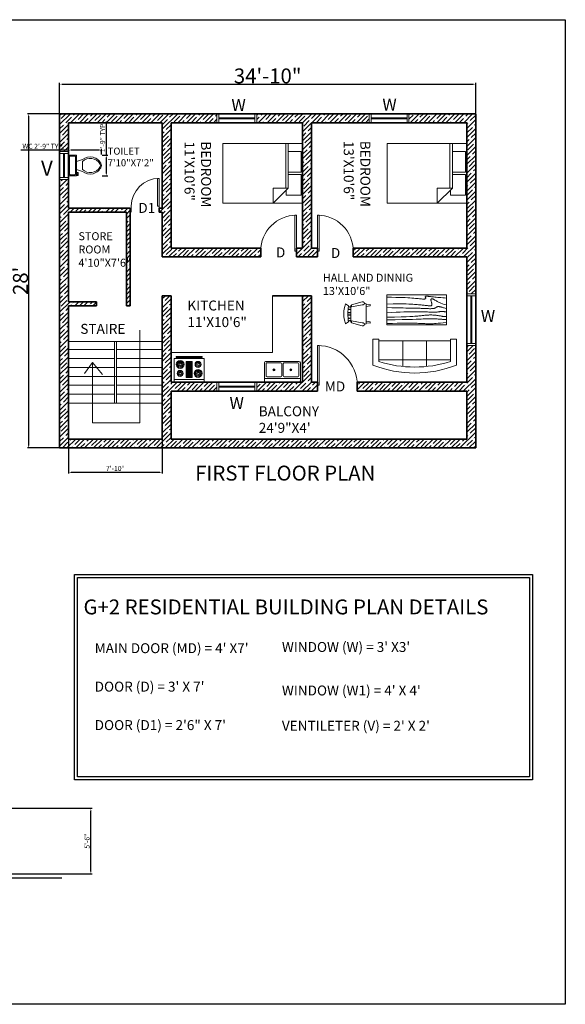
# Model space of a CAD drawing. Units: inches. Extents: x 1662 to 23131, y 1265 to 19127.
# Tile 13 of 26: x 17717 to 18265, y 7742 to 8732. Entities that reach past the tile are written whole.
import ezdxf

# ---------------------------------------------------------------- set-up
doc = ezdxf.new("R2010")
doc.units = ezdxf.units.IN
for name, color, linetype, lineweight in [('A-ANNO-DIMS', 4, 'Continuous', 18), ('A-ANNO-IDEN', 7, 'Continuous', 18), ('A-ANNO-TEXT', 7, 'Continuous', 18), ('A-ANNO-TITL', 7, 'Continuous', 35), ('A-ANNO-TTLB', 7, 'Continuous', 25), ('A-AREA-IDEN', 7, 'Continuous', 18), ('A-DOOR', 3, 'Continuous', 18), ('A-ELEV', 7, 'Continuous', 25), ('A-EQPM', 8, 'Continuous', 18), ('A-FLOR-CASE', 8, 'Continuous', 18), ('A-FLOR-FIXT', 9, 'Continuous', 18), ('A-FLOR-STRS', 7, 'Continuous', 18), ('A-FURN', 8, 'Continuous', 18), ('A-GLAZ', 4, 'Continuous', 18), ('A-WALL', 7, 'Continuous', 35), ('A-WALL-PATT', 8, 'Continuous', 13)]:
    doc.layers.add(name, color=color, linetype=linetype, lineweight=lineweight)
doc.styles.get("Standard").update_dxf_attribs({"font": 'arial.ttf'})
doc.dimstyles.new('ISO-25', dxfattribs={"dimtxt": 5, "dimasz": 2.5, "dimexe": 1.25, "dimexo": 0.625, "dimtad": 1, "dimlunit": 3, "dimtxsty": 'Standard', "dimcen": 2.5, "dimadec": 0, "dimazin": 0, "dimtfac": 1, "dimtmove": 0, "dimatfit": 3, "dimfxl": 1, "dimarcsym": 0})
pattern_1 = [(45, (481.835, -449.725), (-4.490128, 4.490128), []), (45, (486.325, -449.725), (-4.490128, 4.490128), [7.9375, -1.5875, 0, -1.5875])]

# ---------------------------------------------------------------- blocks, each defined once
blk = doc.blocks.new('*U33')
for p, q in [((0, 0), (0, -6)), ((40, 0), (40, -6))]:
    blk.add_line(p, q)
blk.add_lwpolyline([(0, 0), (0, 40), (1.75, 40), (1.75, 0)], close=True)
blk.add_arc((0, 0), 40, 0, 90)
blk = doc.blocks.new('*U69')
for p, q in [((0, 0), (0, -6)), ((36, 0), (36, -6))]:
    blk.add_line(p, q)
blk.add_lwpolyline([(0, 0), (0, 36), (1.75, 36), (1.75, 0)], close=True)
blk.add_arc((0, 0), 36, 0, 90)
blk = doc.blocks.new('*U70')
for p, q in [((0, 0), (0, -6)), ((-36, 0), (-36, -6))]:
    blk.add_line(p, q)
blk.add_lwpolyline([(0, 0), (0, 36), (-1.75, 36), (-1.75, 0)], close=True)
blk.add_arc((0, 0), 36, 90, 180)
blk = doc.blocks.new('*U71')
for p, q in [((-28, 0), (-28, -6)), ((0, 0), (0, -6))]:
    blk.add_line(p, q)
blk.add_lwpolyline([(0, 0), (0, 28), (-1.75, 28), (-1.75, 0)], close=True)
blk.add_arc((0, 0), 28, 90, 180)
blk = doc.blocks.new('Bed - Queen')
for p, q in [((0, -80.00003), (0, 0)), ((0, 0), (59.99999, 0)), ((59.99999, 0), (59.99999, -80.00003)), ((7.99999, -1.2), (28.79998, -1.2)), ((7.99999, -14.4), (7.99999, -1.2)), ((28.79998, -1.2), (28.79998, -14.4)), ((31.19999, -1.2), (51.99999, -1.2)), ((31.19999, -14.4), (31.19999, -1.2)), ((51.99999, -1.2), (51.99999, -16.4)), ((0, -14.4), (44.8, -14.4)), ((44.8, -16.8), (0, -16.8)), ((59.99999, -29.6), (44.8, -14.4)), ((44.8, -14.4), (44.8, -29.6)), ((51.99999, -16.4), (46.79936, -16.4)), ((44.8, -29.6), (59.99999, -29.6)), ((59.99999, -80.00003), (0, -80.00003))]:
    blk.add_line(p, q)
blk = doc.blocks.new('Toilet - top')
for p, q in [((-10, -8.5), (-8, -8.5)), ((-10, -9.5), (-10, -8.5)), ((-7, -9.5), (-10, -9.5)), ((-8, -8.5), (-8, -8)), ((-7, -8), (-7, -9.5)), ((-4, -8), (-6, -14)), ((4, -8), (6, -14)), ((9.5, -6), (9.5, -2)), ((4, -14), (-4, -14))]:
    blk.add_line(p, q)
blk.add_lwpolyline([(10.5, -8), (10.5, 0), (-10.5, 0), (-10.5, -8)], close=True)
for points in [[(-9.5, -2), (-9.5, -6)], [(8.5, -1), (-8.5, -1)], [(-8.5, -7), (8.5, -7)]]:
    blk.add_lwpolyline(points)
for centre, radius, start, end in [((-8.62, -1.88), 0.884, 81.8699, 188.1301), ((-8.62, -6.12), 0.884, 171.8699, 278.1301), ((8.62, -1.88), 0.884, 351.8699, 98.1301), ((8.62, -6.12), 0.884, 261.8699, 8.1301), ((3.52, -21.58), 12.17, 141.46911, 247.97143), ((4.2, -21.82), 11.33, 136.36773, 238.94682), ((-3.52, -21.58), 12.17, 292.02843, 38.53071), ((-4.2, -21.82), 11.33, 301.05301, 43.63209), ((0, -27.88), 4, 245.73182, 294.26817), ((0, -29), 4, 254.86053, 285.13947)]:
    blk.add_arc(centre, radius, start, end)
blk = doc.blocks.new('Range-Oven - 30 in top')
for p, q in [((0, -3), (30, -3)), ((12, -6), (18, -6)), ((13, -20), (13, -6)), ((14, -6), (14, -20)), ((15, -20), (15, -6)), ((16, -6), (16, -20)), ((17, -20), (17, -6)), ((6, -24), (6, -25)), ((8, -25), (8, -24)), ((18, -20), (12, -20)), ((22, -25), (22, -24)), ((24, -24), (24, -25))]:
    blk.add_line(p, q)
for points in [[(0, -24), (0, 0), (30, 0), (30, -24)], [(12, -21), (12, -5), (18, -5), (18, -21)], [(2, -26), (2, -25), (28, -25), (28, -26)]]:
    blk.add_lwpolyline(points, close=True)
for centre, radius in [((6, -9), 4), ((6, -9), 3), ((6, -9), 2), ((6, -9), 1), ((24, -9), 3), ((24, -9), 2), ((24, -9), 1), ((6, -18), 3), ((6, -18), 2), ((6, -18), 1), ((24, -18), 4), ((24, -18), 3), ((24, -18), 2), ((24, -18), 1)]:
    blk.add_circle(centre, radius)
blk = doc.blocks.new('Sink-double - 36 in top')
for p, q in [((-18, -4), (18, -4)), ((-0.75, -18.5), (-0.75, -6.5)), ((0.75, -6.5), (0.75, -18.5))]:
    blk.add_line(p, q)
for points in [[(-16.5, 0), (16.5, 0)], [(-18, -19.5), (-18, -1.5)], [(-16.5, -18.5), (-16.5, -6.5)], [(-15.5, -5.5), (-1.75, -5.5)], [(1.75, -5.5), (15.5, -5.5)], [(16.5, -6.5), (16.5, -18.5)], [(18, -1.5), (18, -19.5)], [(-1.75, -19.5), (-15.5, -19.5)], [(15.5, -19.5), (1.75, -19.5)], [(16.5, -21), (-16.5, -21)]]:
    blk.add_lwpolyline(points)
for centre, radius in [((-8.5, -12.5), 1), ((-8.5, -12.5), 0.5), ((8.5, -12.5), 1), ((8.5, -12.5), 0.5)]:
    blk.add_circle(centre, radius)
for centre, radius, start, end in [((-16.5, -1.5), 1.5, 90, 180), ((16.5, -1.5), 1.5, 0, 90), ((-15.5, -6.5), 1, 90, 180), ((-1.75, -6.5), 1, 0, 90), ((1.75, -6.5), 1, 90, 180), ((15.5, -6.5), 1, 0, 90), ((-16.5, -19.5), 1.5, 180, 270), ((-15.5, -18.5), 1, 180, 270), ((-1.75, -18.5), 1, 270, 0), ((1.75, -18.5), 1, 180, 270), ((15.5, -18.5), 1, 270, 0), ((16.5, -19.5), 1.5, 270, 0)]:
    blk.add_arc(centre, radius, start, end)
blk = doc.blocks.new('Sofa - Roundback 7 ft.')
for p, q in [((-12.00002, -32.4421), (-12.00003, -6.5971)), ((11.99997, -32.4421), (11.99998, -6.5971)), ((-36.000027, -34), (-36.000027, -11.4696)), ((-35.999844, -13.3819), (35.9998, -13.3819)), ((35.99998, -34), (35.99998, -11.4696)), ((-36.000027, -32.4421), (35.99998, -32.4421))]:
    blk.add_line(p, q)
for points in [[(-36.000027, -34), (-42.000027, -34), (-42.000027, -8)], [(41.99998, -8), (41.99998, -34), (35.99998, -34)]]:
    blk.add_lwpolyline(points)
for centre, radius, start, end in [((0, -114.25), 114.25, 68.43141, 111.5686), ((-0.00001, -127.1968), 121.1968, 72.72033, 107.2797)]:
    blk.add_arc(centre, radius, start, end)
blk = doc.blocks.new('Table - Rectangular Woodgrain 60 x 30 in.')
for p, q in [((0, 0), (0, -30)), ((60, 0), (0, 0)), ((60, -30), (60, 0)), ((0, -30), (60, -30))]:
    blk.add_line(p, q)
for points in [[(0, -2.4), (4.8155, -2.418), (9.0302, -2.4688), (12.709, -2.5477), (15.9167, -2.65), (18.7181, -2.7711), (21.1781, -2.9063), (23.3616, -3.0508), (25.3333, -3.2), (27.1477, -3.3495), (28.8172, -3.4958), (30.3437, -3.636), (31.7291, -3.7667), (32.9756, -3.8849), (34.0849, -3.9875), (35.059, -4.0714), (35.9, -4.1334), (36.6114, -4.1711), (37.2041, -4.1854), (37.6906, -4.1779), (38.0833, -4.15), (38.3948, -4.1034), (38.6375, -4.0396), (38.8239, -3.9602), (38.9666, -3.8667), (39.0764, -3.7608), (39.1573, -3.6448), (39.2116, -3.521), (39.2416, -3.3917), (39.2498, -3.2593), (39.2385, -3.1261), (39.21, -2.9944), (39.1666, -2.8667), (39.111, -2.7447), (39.0468, -2.6281), (38.978, -2.5163), (38.9083, -2.4083), (38.8418, -2.3035), (38.7823, -2.201), (38.7337, -2.1001), (38.7, -2), (38.6844, -1.9003), (38.6875, -1.8021), (38.7094, -1.707), (38.75, -1.6167), (38.8094, -1.5326), (38.8875, -1.4563), (38.9844, -1.3893), (39.1, -1.3333), (39.2351, -1.2896), (39.3937, -1.2583), (39.5804, -1.2396), (39.8, -1.2333), (40.057, -1.2396), (40.3562, -1.2583), (40.7023, -1.2896), (41.1, -1.3333), (41.5547, -1.3895), (42.0755, -1.4573), (42.6721, -1.5361), (43.3542, -1.625), (44.1316, -1.7233), (45.014, -1.8302), (46.0114, -1.9449), (47.1333, -2.0667), (48.3862, -2.1947), (49.7625, -2.3281), (51.2513, -2.4663), (52.8416, -2.6083), (54.5226, -2.7535), (56.2833, -2.9011), (58.1127, -3.0501), (60, -3.2)], [(0, -9.2), (6.5759, -9.0858), (11.9385, -9.0365), (16.2527, -9.0418), (19.6833, -9.0917), (22.3952, -9.1759), (24.5531, -9.2844), (26.322, -9.4069), (27.8666, -9.5333), (29.3241, -9.6553), (30.7203, -9.7719), (32.0532, -9.8837), (33.3208, -9.9917), (34.5213, -10.0965), (35.6526, -10.199), (36.7128, -10.2999), (37.7, -10.4), (38.6129, -10.4996), (39.4531, -10.5969), (40.223, -10.6895), (40.925, -10.775), (41.5613, -10.8512), (42.1344, -10.9156), (42.6465, -10.966), (43.1, -11), (43.4976, -11.0158), (43.8437, -11.0136), (44.143, -10.9942), (44.4, -10.9583), (44.6195, -10.9069), (44.8062, -10.8406), (44.9648, -10.7603), (45.1, -10.6667), (45.2155, -10.5598), (45.3114, -10.4365), (45.3871, -10.2929), (45.4416, -10.125), (45.4743, -9.929), (45.4844, -9.7011), (45.4709, -9.4371), (45.4333, -9.1333), (45.3716, -8.7883), (45.2896, -8.4104), (45.1919, -8.0107), (45.0833, -7.6), (44.9685, -7.1893), (44.8521, -6.7896), (44.7388, -6.4117), (44.6333, -6.0667), (44.54, -5.7628), (44.4614, -5.4979), (44.4001, -5.2675), (44.3583, -5.0667), (44.3384, -4.8909), (44.3427, -4.7354), (44.3736, -4.5956), (44.4333, -4.4667), (44.5236, -4.3453), (44.6427, -4.2333), (44.7884, -4.1339), (44.9583, -4.05), (45.1501, -3.9849), (45.3614, -3.9417), (45.59, -3.9234), (45.8333, -3.9333), (46.0915, -3.9749), (46.3734, -4.0531), (46.6906, -4.1736), (47.0542, -4.3417), (47.4756, -4.5629), (47.9661, -4.8427), (48.5372, -5.1866), (49.2, -5.6), (49.9676, -6.0844), (50.8594, -6.625), (51.8965, -7.2031), (53.1, -7.8), (54.491, -8.3969), (56.0906, -8.975), (57.9199, -9.5156), (60, -10)], [(0, -12.8), (5.1847, -12.9322), (9.6213, -13.0323), (13.3963, -13.1059), (16.5958, -13.1583), (19.3063, -13.1952), (21.614, -13.2219), (23.6054, -13.2439), (25.3666, -13.2667), (26.9728, -13.2947), (28.4531, -13.3281), (29.8256, -13.3663), (31.1083, -13.4083), (32.3191, -13.4535), (33.476, -13.501), (34.597, -13.5501), (35.7, -13.6), (36.7984, -13.6497), (37.8875, -13.6979), (38.9578, -13.743), (40, -13.7833), (41.0047, -13.8174), (41.9625, -13.8438), (42.864, -13.8607), (43.7, -13.8667), (44.4631, -13.8604), (45.1552, -13.8417), (45.7801, -13.8104), (46.3416, -13.7667), (46.8439, -13.7104), (47.2906, -13.6417), (47.6858, -13.5604), (48.0333, -13.4667), (48.3375, -13.3608), (48.6042, -13.2448), (48.8396, -13.121), (49.05, -12.9917), (49.2417, -12.8593), (49.4208, -12.7261), (49.5937, -12.5944), (49.7667, -12.4667), (49.9452, -12.3451), (50.1323, -12.2313), (50.3303, -12.1268), (50.5416, -12.0333), (50.7686, -11.9524), (51.0135, -11.8854), (51.2788, -11.8341), (51.5666, -11.8), (51.8785, -11.7843), (52.2116, -11.7865), (52.562, -11.8059), (52.926, -11.8417), (53.2998, -11.8931), (53.6795, -11.9594), (54.0614, -12.0397), (54.4416, -12.1333), (54.8223, -12.2401), (55.2293, -12.3625), (55.6942, -12.5037), (56.2489, -12.6667), (56.9251, -12.8547), (57.7545, -13.0708), (58.7689, -13.3182), (60, -13.6)], [(0, -18), (5.124, -17.7273), (9.6609, -17.5057), (13.6705, -17.3303), (17.2125, -17.1958), (20.3467, -17.0973), (23.1328, -17.0297), (25.6307, -16.9878), (27.9, -16.9667), (29.9928, -16.9617), (31.9302, -16.9703), (33.7254, -16.9907), (35.3917, -17.0208), (36.9423, -17.0588), (38.3906, -17.1026), (39.7499, -17.1503), (41.0333, -17.2), (42.2519, -17.2496), (43.4073, -17.2969), (44.4986, -17.3395), (45.525, -17.375), (46.4858, -17.4012), (47.3802, -17.4156), (48.2074, -17.416), (48.9667, -17.4), (49.6583, -17.3662), (50.2872, -17.3167), (50.8595, -17.2547), (51.3812, -17.1833), (51.8584, -17.1057), (52.2971, -17.025), (52.7034, -16.9443), (53.0833, -16.8667), (53.443, -16.7951), (53.789, -16.7313), (54.128, -16.6768), (54.4666, -16.6334), (54.8115, -16.6024), (55.1693, -16.5854), (55.5465, -16.5841), (55.95, -16.6), (56.3828, -16.6337), (56.8346, -16.6823), (57.2915, -16.7418), (57.7396, -16.8084), (58.165, -16.878), (58.5539, -16.9469), (58.8924, -17.0111), (59.1666, -17.0667), (59.3679, -17.1107), (59.5078, -17.1438), (59.6032, -17.1675), (59.6708, -17.1833), (59.7275, -17.193), (59.7901, -17.1979), (59.8753, -17.1998), (60, -17.2)], [(0, -22.4), (8.0098, -22.2501), (14.4094, -22.1011), (19.4168, -21.9535), (23.25, -21.8083), (26.1269, -21.6663), (28.2656, -21.5281), (29.884, -21.3947), (31.2, -21.2667), (32.3967, -21.1448), (33.5172, -21.0292), (34.5697, -20.9198), (35.5625, -20.8167), (36.5037, -20.7198), (37.4015, -20.6292), (38.2642, -20.5448), (39.1, -20.4667), (39.9164, -20.3951), (40.7187, -20.3313), (41.5117, -20.2768), (42.3, -20.2333), (43.0883, -20.2024), (43.8812, -20.1854), (44.6836, -20.1841), (45.5, -20.2), (46.3328, -20.234), (47.1747, -20.2844), (48.0163, -20.3488), (48.8479, -20.425), (49.66, -20.5106), (50.4429, -20.6031), (51.1872, -20.7004), (51.8833, -20.8), (52.5246, -20.8999), (53.1166, -20.9995), (53.6681, -21.0983), (54.1875, -21.1958), (54.6834, -21.2919), (55.1646, -21.3859), (55.6394, -21.4777), (56.1167, -21.5667), (56.6028, -21.6515), (57.0961, -21.7266), (57.5929, -21.7852), (58.0896, -21.8208), (58.5823, -21.8268), (59.0674, -21.7964), (59.5412, -21.723), (60, -21.6)], [(0, -25.2), (8.6355, -25.0504), (15.7026, -24.9031), (21.4049, -24.7606), (25.9458, -24.625), (29.529, -24.4988), (32.3578, -24.3844), (34.6359, -24.284), (36.5667, -24.2), (38.3213, -24.1341), (39.9417, -24.0854), (41.437, -24.0523), (42.8167, -24.0333), (44.0901, -24.0268), (45.2667, -24.0313), (46.3557, -24.0451), (47.3667, -24.0667), (48.309, -24.0947), (49.1928, -24.1287), (50.0284, -24.168), (50.826, -24.2125), (51.5959, -24.2617), (52.3483, -24.3151), (53.0935, -24.3725), (53.8417, -24.4334), (54.6009, -24.497), (55.3699, -24.561), (56.1454, -24.6226), (56.9239, -24.6792), (57.7021, -24.7279), (58.4764, -24.7662), (59.2435, -24.7911), (60, -24.8)], [(0, -28.8), (5.6867, -28.6681), (10.45, -28.5698), (14.407, -28.5012), (17.675, -28.4584), (20.3711, -28.4374), (22.6125, -28.4344), (24.5164, -28.4455), (26.2, -28.4667), (27.762, -28.4947), (29.2276, -28.5281), (30.6033, -28.5663), (31.8958, -28.6084), (33.1118, -28.6535), (34.2578, -28.7011), (35.3405, -28.7501), (36.3666, -28.8), (37.3443, -28.8497), (38.288, -28.8974), (39.2137, -28.9412), (40.1375, -28.9792), (41.0753, -29.0093), (42.0432, -29.0297), (43.0572, -29.0384), (44.1333, -29.0333), (45.2936, -29.0114), (46.5843, -28.9641), (48.0579, -28.8816), (49.7666, -28.7542), (51.7629, -28.5721), (54.0989, -28.3255), (56.8272, -28.0048), (60, -27.6)]]:
    blk.add_lwpolyline(points)
blk = doc.blocks.new('Chair - Rocking')
for p, q in [((-9, -7.5), (-12, -18.49999)), ((-8, -4.5), (-10, -1.5)), ((-7, -7.5), (-9, -7.5)), ((-9, -18.49999), (-7, -7.5)), ((-8.23428, -6.99939), (-8.3093, -7.47958)), ((-8.23041, -7), (8.23915, -7)), ((-7.5, -4.5), (-7, -7)), ((-6.5, -7), (-7.02225, -4.43)), ((-4.5, -7), (-4.96674, -4.19951)), ((-4, -7), (-4.40532, -4.16272)), ((-1.5, -4.05012), (-1.5, -7)), ((-1, -7), (-1, -4.05012)), ((1, -7), (1, -4.04655)), ((1.5, -4.05012), (1.5, -7)), ((4, -7), (4.40187, -4.18694)), ((4.5, -7), (4.96761, -4.19437)), ((6.5, -7), (7, -4.4057)), ((7.5, -4.5), (7, -7)), ((7, -7.5), (9, -7.5)), ((9, -18.49999), (7, -7.5)), ((8, -4.5), (10, -1.5)), ((8.31071, -7.48854), (8.23449, -7.00073)), ((9, -7.5), (12, -18.49999)), ((-10.36644, -20.64523), (-10.5, -21.49999)), ((-9, -22.49999), (-9.5, -26.49999)), ((0, -22.49999), (-9.5, -22.49999)), ((-9.5, -26.49999), (-8, -26.49999)), ((-8, -26.49999), (-7.5, -22.49999)), ((0, -22.49999), (9.5, -22.49999)), ((8, -26.49999), (7.5, -22.49999)), ((9.5, -26.49999), (8, -26.49999)), ((9, -22.49999), (9.5, -26.49999)), ((10.5, -21.49999), (10.3575, -20.58798))]:
    blk.add_line(p, q)
for centre, radius, start, end in [((0, -34.08333), 34.08333, 72.93847, 107.0615), ((0, -68.25004), 64.25, 93.92211, 97.15267), ((0, -68.25004), 64.25, 82.84733, 93.92211), ((-10.5, -18.99999), 1.58114, 161.5651, 18.43495), ((10.5, -18.99999), 1.58114, 161.5651, 18.43495), ((-9.5, -21.49999), 1, 180, 270), ((9.5, -21.49999), 1, 270, 0)]:
    blk.add_arc(centre, radius, start, end)
blk = doc.blocks.new('*D74')
at = {"layer": 'A-ANNO-DIMS', "color": 0, "lineweight": -2, "transparency": 16777216}
for p, q in [((17756.47, 8637.39), (17724.69, 8637.39)), ((17725.94, 8634.89), (17725.94, 8303.89)), ((17756.47, 8301.39), (17724.69, 8301.39))]:
    blk.add_line(p, q, dxfattribs=at)
at = {"layer": 'A-ANNO-DIMS', "color": 0, "transparency": 16777216}
for points in [[(17725.53, 8634.89), (17726.36, 8634.89), (17725.94, 8637.39)], [(17725.53, 8303.89), (17726.36, 8303.89), (17725.94, 8301.39)]]:
    blk.add_solid(points, dxfattribs=at)
at = {"layer": 'Defpoints', "color": 0, "transparency": 16777216}
for p in [(17757.09, 8637.39), (17725.94, 8301.39), (17757.09, 8301.39)]:
    blk.add_point(p, dxfattribs=at)
at = {"layer": 'A-ANNO-DIMS', "color": 0, "transparency": 16777216, "insert": (17717.66, 8469.39), "char_height": 5, "attachment_point": 5, "rotation": 90}
blk.add_mtext("{\\H3x;28'}", dxfattribs=at)
blk = doc.blocks.new('*D75')
at = {"layer": 'A-ANNO-DIMS', "color": 0, "lineweight": -2, "transparency": 16777216}
for p, q in [((17757.09, 8638.02), (17757.09, 8668.36)), ((17759.59, 8667.11), (18172.59, 8667.11)), ((18175.09, 8638.02), (18175.09, 8668.36))]:
    blk.add_line(p, q, dxfattribs=at)
at = {"layer": 'A-ANNO-DIMS', "color": 0, "transparency": 16777216}
for points in [[(17759.59, 8667.52), (17759.59, 8666.69), (17757.09, 8667.11)], [(18172.59, 8667.52), (18172.59, 8666.69), (18175.09, 8667.11)]]:
    blk.add_solid(points, dxfattribs=at)
at = {"layer": 'Defpoints', "color": 0, "transparency": 16777216}
for p in [(18175.09, 8667.11), (17757.09, 8637.39), (18175.09, 8637.39)]:
    blk.add_point(p, dxfattribs=at)
at = {"layer": 'A-ANNO-DIMS', "color": 0, "transparency": 16777216, "insert": (17966.09, 8675.39), "char_height": 5, "attachment_point": 5}
blk.add_mtext('{\\H3x;34\'-10"}', dxfattribs=at)
blk = doc.blocks.new('SCHEDULE-FRAME')
for points in [[(0, 206.36), (460.01, 206.36), (460.01, 0), (0, 0)], [(3, 203.36), (457.01, 203.36), (457.01, 3), (3, 3)]]:
    blk.add_lwpolyline(points, close=True)
blk = doc.blocks.new('*D161')
at = {"layer": 'A-ANNO-DIMS', "color": 0, "lineweight": -2, "transparency": 16777216}
for p, q in [((17766.09, 8596.52), (17766.09, 8602.1)), ((17799.14, 8596.52), (17799.14, 8602.1)), ((17766.09, 8600.85), (17718.08, 8600.85)), ((17796.64, 8600.85), (17768.59, 8600.85))]:
    blk.add_line(p, q, dxfattribs=at)
at = {"layer": 'A-ANNO-DIMS', "color": 0, "transparency": 16777216}
for points in [[(17768.59, 8601.27), (17768.59, 8600.43), (17766.09, 8600.85)], [(17796.64, 8601.27), (17796.64, 8600.43), (17799.14, 8600.85)]]:
    blk.add_solid(points, dxfattribs=at)
at = {"layer": 'Defpoints', "color": 0, "transparency": 16777216}
for p in [(17766.09, 8600.85), (17766.09, 8595.89), (17799.14, 8595.89)]:
    blk.add_point(p, dxfattribs=at)
at = {"layer": 'A-ANNO-DIMS', "color": 0, "transparency": 16777216, "insert": (17740.84, 8604.06), "char_height": 5, "attachment_point": 5}
blk.add_mtext('WC 2\'-9" TYP.', dxfattribs=at)
blk = doc.blocks.new('*D162')
at = {"layer": 'A-ANNO-DIMS', "color": 0, "lineweight": -2, "transparency": 16777216}
for p, q in [((17804.1, 8595.89), (17804.1, 8629.65)), ((17799.76, 8595.89), (17805.35, 8595.89)), ((17804.1, 8577.39), (17804.1, 8593.39)), ((17799.76, 8574.89), (17805.35, 8574.89))]:
    blk.add_line(p, q, dxfattribs=at)
at = {"layer": 'A-ANNO-DIMS', "color": 0, "transparency": 16777216}
for points in [[(17803.68, 8593.39), (17804.51, 8593.39), (17804.1, 8595.89)], [(17803.68, 8577.39), (17804.51, 8577.39), (17804.1, 8574.89)]]:
    blk.add_solid(points, dxfattribs=at)
at = {"layer": 'Defpoints', "color": 0, "transparency": 16777216}
for p in [(17799.14, 8595.89), (17804.1, 8595.89), (17799.14, 8574.89)]:
    blk.add_point(p, dxfattribs=at)
at = {"layer": 'A-ANNO-DIMS', "color": 0, "transparency": 16777216, "insert": (17800.92, 8614.02), "char_height": 5, "attachment_point": 5, "rotation": 90}
blk.add_mtext('1\'-9" TYP.', dxfattribs=at)
blk = doc.blocks.new('*D229')
at = {"layer": 'A-ANNO-DIMS', "color": 0, "lineweight": -2, "transparency": 16777216}
for p, q in [((17766.09, 8309.77), (17766.09, 8275.74)), ((17860.09, 8309.77), (17860.09, 8275.74)), ((17768.59, 8276.99), (17857.59, 8276.99))]:
    blk.add_line(p, q, dxfattribs=at)
at = {"layer": 'A-ANNO-DIMS', "color": 0, "transparency": 16777216}
for points in [[(17768.59, 8277.41), (17768.59, 8276.58), (17766.09, 8276.99)], [(17857.59, 8277.41), (17857.59, 8276.58), (17860.09, 8276.99)]]:
    blk.add_solid(points, dxfattribs=at)
at = {"layer": 'Defpoints', "color": 0, "transparency": 16777216}
for p in [(17766.09, 8310.39), (17860.09, 8310.39), (17860.09, 8276.99)]:
    blk.add_point(p, dxfattribs=at)
at = {"layer": 'A-ANNO-DIMS', "color": 0, "transparency": 16777216, "insert": (17813.09, 8280.17), "char_height": 5, "attachment_point": 5}
blk.add_mtext('7\'-10"', dxfattribs=at)
blk = doc.blocks.new('*D238')
at = {"layer": 'A-ANNO-DIMS', "color": 0, "lineweight": -2, "transparency": 16777216}
for p, q in [((17585.88, 7939.16), (17789.71, 7939.16)), ((17788.46, 7875.66), (17788.46, 7936.66)), ((17585.88, 7873.16), (17789.71, 7873.16))]:
    blk.add_line(p, q, dxfattribs=at)
at = {"layer": 'A-ANNO-DIMS', "color": 0, "transparency": 16777216}
for points in [[(17788.04, 7936.66), (17788.87, 7936.66), (17788.46, 7939.16)], [(17788.04, 7875.66), (17788.87, 7875.66), (17788.46, 7873.16)]]:
    blk.add_solid(points, dxfattribs=at)
at = {"layer": 'Defpoints', "color": 0, "transparency": 16777216}
for p in [(17585.26, 7939.16), (17788.46, 7939.16), (17585.26, 7873.16)]:
    blk.add_point(p, dxfattribs=at)
at = {"layer": 'A-ANNO-DIMS', "color": 0, "transparency": 16777216, "insert": (17785.28, 7906.16), "char_height": 5, "attachment_point": 5, "rotation": 90}
blk.add_mtext('5\'-6"', dxfattribs=at)

msp = doc.modelspace()

# ---------------------------------------------------------------- hatches: boundary and pattern name
at = {"layer": 'A-WALL-PATT'}
h = msp.add_hatch(dxfattribs=at)
h.set_pattern_fill('ANSI35', color=256)
h.set_pattern_definition(pattern_1)
h.paths.add_polyline_path([(17757.093, 8301.392), (18175.093, 8301.392), (18175.093, 8404.392), (18166.093, 8404.392), (18166.093, 8367.392), (18056.093, 8367.392), (18056.093, 8358.392), (18166.093, 8358.392), (18166.093, 8310.392), (17869.093, 8310.392), (17869.093, 8358.392), (17915.093, 8358.392), (17915.093, 8367.392), (17869.093, 8367.392), (17869.093, 8454.392), (17860.093, 8454.392), (17860.093, 8310.392), (17766.093, 8310.392), (17766.093, 8444.392), (17794.093, 8444.392), (17794.093, 8448.392), (17766.093, 8448.392), (17766.093, 8538.392), (17824.093, 8538.392), (17824.093, 8444.392), (17828.093, 8444.392), (17828.093, 8542.392), (17766.093, 8542.392), (17766.093, 8571.392), (17757.093, 8571.392)])
h.paths.add_polyline_path([(17959.093, 8493.392), (17959.093, 8502.392), (17869.093, 8502.392), (17869.093, 8628.392), (17915.093, 8628.392), (17915.093, 8637.392), (17757.093, 8637.392), (17757.093, 8599.392), (17766.093, 8599.392), (17766.093, 8628.392), (17860.093, 8628.392), (17860.093, 8542.392), (17857.093, 8542.392), (17857.093, 8538.392), (17860.093, 8538.392), (17860.093, 8493.392)])
h.paths.add_polyline_path([(18016.093, 8493.392), (18016.093, 8502.392), (18010.093, 8502.392), (18010.093, 8628.392), (18068.093, 8628.392), (18068.093, 8637.392), (17955.093, 8637.392), (17955.093, 8628.392), (18001.093, 8628.392), (18001.093, 8502.392), (17995.093, 8502.392), (17995.093, 8493.392)])
h.paths.add_polyline_path([(18052.093, 8502.392), (18052.093, 8493.392), (18166.093, 8493.392), (18166.093, 8456.392), (18175.093, 8456.392), (18175.093, 8637.392), (18108.093, 8637.392), (18108.093, 8628.392), (18166.093, 8628.392), (18166.093, 8502.392)])
h.paths.add_polyline_path([(17773.079, 8478.929), (17828.549, 8478.929), (17828.549, 8522.256), (17773.079, 8522.256)], flags=25)
h = msp.add_hatch(dxfattribs=at)
h.set_pattern_fill('ANSI35', color=256)
h.set_pattern_definition(pattern_1)
h.paths.add_polyline_path([(18016.093, 8358.392), (18016.093, 8364.392), (18016.093, 8367.392), (18010.093, 8367.392), (18010.093, 8454.392), (18001.093, 8454.392), (18001.093, 8367.392), (17955.093, 8367.392), (17955.093, 8358.392)])

# ---------------------------------------------------------------- linework, layer by layer
at = {"layer": 'A-ANNO-TTLB'}
msp.add_lwpolyline([(17164.976, 8731.935), (18265.142, 8731.935), (18265.142, 7742.121), (17164.976, 7742.121)], close=True, dxfattribs=at)
at = {"layer": 'A-ELEV'}
msp.add_line((17693.258, 7869.159), (17759.108, 7869.159), dxfattribs=at)
at = {"layer": 'A-FLOR-CASE'}
for p in [(17971.093, 8454.392), (17869.093, 8397.392)]:
    msp.add_line(p, (17971.093, 8397.392), dxfattribs=at)
at = {"layer": 'A-FLOR-STRS'}
for p, q in [((17837.614, 8419.922), (17837.614, 8326.609)), ((17766.093, 8408.392), (17860.093, 8408.392)), ((17812.093, 8346.392), (17812.093, 8408.392)), ((17814.093, 8346.392), (17814.093, 8408.392)), ((17812.093, 8400.392), (17766.093, 8400.392)), ((17860.093, 8400.392), (17814.093, 8400.392)), ((17812.093, 8391.392), (17766.093, 8391.392)), ((17790.064, 8387.416), (17781.96, 8376.206)), ((17790.064, 8326.609), (17790.064, 8387.416)), ((17790.064, 8387.416), (17800.071, 8375.396)), ((17860.093, 8391.392), (17814.093, 8391.392)), ((17812.093, 8382.392), (17766.093, 8382.392)), ((17860.093, 8382.392), (17814.093, 8382.392)), ((17860.093, 8373.392), (17766.093, 8373.392)), ((17812.093, 8364.392), (17766.093, 8364.392)), ((17860.093, 8364.392), (17814.093, 8364.392)), ((17812.093, 8355.392), (17766.093, 8355.392)), ((17860.093, 8355.392), (17814.093, 8355.392)), ((17860.093, 8346.392), (17766.093, 8346.392)), ((17837.614, 8326.609), (17790.064, 8326.609))]:
    msp.add_line(p, q, dxfattribs=at)
at = {"layer": 'A-GLAZ'}
for p, q in [((17915.093, 8628.392), (17915.093, 8637.392)), ((17917.093, 8628.392), (17917.093, 8637.392)), ((17953.093, 8633.392), (17917.093, 8633.392)), ((17953.093, 8632.892), (17917.093, 8632.892)), ((17953.093, 8632.392), (17917.093, 8632.392)), ((17953.093, 8628.392), (17953.093, 8637.392)), ((17955.093, 8628.392), (17955.093, 8637.392)), ((18068.093, 8628.392), (18068.093, 8637.392)), ((18070.093, 8628.392), (18070.093, 8637.392)), ((18106.093, 8633.392), (18070.093, 8633.392)), ((18106.093, 8632.892), (18070.093, 8632.892)), ((18106.093, 8632.392), (18070.093, 8632.392)), ((18106.093, 8628.392), (18106.093, 8637.392)), ((18108.093, 8628.392), (18108.093, 8637.392)), ((17766.093, 8599.392), (17757.093, 8599.392)), ((17766.093, 8597.392), (17757.093, 8597.392)), ((17761.093, 8597.392), (17761.093, 8573.392)), ((17761.593, 8597.392), (17761.593, 8573.392)), ((17762.093, 8597.392), (17762.093, 8573.392)), ((17766.093, 8573.392), (17757.093, 8573.392)), ((17766.093, 8571.392), (17757.093, 8571.392)), ((18175.093, 8456.392), (18166.093, 8456.392)), ((18175.093, 8454.392), (18166.093, 8454.392)), ((18170.093, 8454.392), (18170.093, 8406.392)), ((18170.593, 8454.392), (18170.593, 8406.392)), ((18171.093, 8454.392), (18171.093, 8406.392)), ((18175.093, 8406.392), (18166.093, 8406.392)), ((18175.093, 8404.392), (18166.093, 8404.392)), ((17915.093, 8358.392), (17915.093, 8367.392)), ((17917.093, 8358.392), (17917.093, 8367.392)), ((17953.093, 8358.392), (17953.093, 8367.392)), ((17955.093, 8358.392), (17955.093, 8367.392)), ((17953.093, 8363.392), (17917.093, 8363.392)), ((17953.093, 8362.892), (17917.093, 8362.892)), ((17953.093, 8362.392), (17917.093, 8362.392))]:
    msp.add_line(p, q, dxfattribs=at)
at = {"layer": 'A-WALL'}
for p, q in [((17757.093, 8637.392), (17757.093, 8301.392)), ((17757.093, 8637.392), (18175.093, 8637.392)), ((18175.093, 8637.392), (18175.093, 8301.392)), ((17766.093, 8628.392), (17860.093, 8628.392)), ((17766.093, 8628.392), (17766.093, 8542.392)), ((17860.093, 8628.392), (17860.093, 8542.392)), ((17869.093, 8628.392), (17869.093, 8502.392)), ((17869.093, 8628.392), (18001.093, 8628.392)), ((18001.093, 8628.392), (18001.093, 8502.392)), ((18010.093, 8628.392), (18010.093, 8502.392)), ((18010.093, 8628.392), (18166.093, 8628.392)), ((18166.093, 8628.392), (18166.093, 8502.392)), ((17766.093, 8542.392), (17828.093, 8542.392)), ((17828.093, 8542.392), (17828.093, 8444.392)), ((17857.093, 8542.392), (17857.093, 8538.392)), ((17857.093, 8542.392), (17860.093, 8542.392)), ((17766.093, 8538.392), (17824.093, 8538.392)), ((17766.093, 8538.392), (17766.093, 8448.392)), ((17824.093, 8538.392), (17824.093, 8444.392)), ((17857.093, 8538.392), (17860.093, 8538.392)), ((17860.093, 8538.392), (17860.093, 8493.392)), ((17860.093, 8493.392), (17959.093, 8493.392)), ((17869.093, 8502.392), (17959.093, 8502.392)), ((17959.093, 8502.392), (17959.093, 8493.392)), ((17995.093, 8502.392), (17995.093, 8493.392)), ((17995.093, 8502.392), (18001.093, 8502.392)), ((17995.093, 8493.392), (18016.093, 8493.392)), ((18010.093, 8502.392), (18016.093, 8502.392)), ((18016.093, 8502.392), (18016.093, 8493.392)), ((18052.093, 8502.392), (18052.093, 8493.392)), ((18052.093, 8502.392), (18166.093, 8502.392)), ((18052.093, 8493.392), (18166.093, 8493.392)), ((18166.093, 8493.392), (18166.093, 8367.392)), ((17869.093, 8454.392), (17860.093, 8454.392)), ((17860.093, 8454.392), (17860.093, 8310.392)), ((17869.093, 8454.392), (17869.093, 8367.392)), ((17971.093, 8454.392), (18010.093, 8454.392)), ((18001.093, 8454.392), (18001.093, 8367.392)), ((18010.093, 8454.392), (18010.093, 8367.392)), ((17766.093, 8448.392), (17794.093, 8448.392)), ((17766.093, 8444.392), (17794.093, 8444.392)), ((17766.093, 8444.392), (17766.093, 8310.392)), ((17794.093, 8448.392), (17794.093, 8444.392)), ((17824.093, 8444.392), (17828.093, 8444.392)), ((17869.093, 8367.392), (18001.093, 8367.392)), ((18010.093, 8367.392), (18016.093, 8367.392)), ((18016.093, 8367.392), (18016.093, 8358.392)), ((18056.093, 8367.392), (18056.093, 8358.392)), ((18056.093, 8367.392), (18166.093, 8367.392)), ((17869.093, 8358.392), (18016.093, 8358.392)), ((17869.093, 8358.392), (17869.093, 8310.392)), ((18056.093, 8358.392), (18166.093, 8358.392)), ((18166.093, 8358.392), (18166.093, 8310.392)), ((17766.093, 8310.392), (17860.093, 8310.392)), ((17860.093, 8310.392), (17766.093, 8310.392)), ((18166.093, 8310.392), (17869.093, 8310.392)), ((18175.093, 8301.392), (17757.093, 8301.392))]:
    msp.add_line(p, q, dxfattribs=at)

# ---------------------------------------------------------------- block references
at = {"layer": 'A-ANNO-TTLB'}
msp.add_blockref('SCHEDULE-FRAME', (17772.134, 7967.79), dxfattribs=at)
at = {"layer": 'A-DOOR'}
for name, p in [('*U71', (17857.093, 8544.392)), ('*U70', (17995.093, 8499.392)), ('*U69', (18016.093, 8499.392)), ('*U33', (18016.093, 8364.392))]:
    msp.add_blockref(name, p, dxfattribs=at)
at = {"layer": 'A-EQPM', "rotation": 180}
msp.add_blockref('Range-Oven - 30 in top', (17902.164, 8367.392), dxfattribs=at)
at = {"layer": 'A-FLOR-FIXT'}
for name, p, rotation in [('Toilet - top', (17766.093, 8585.392), 90), ('Sink-double - 36 in top', (17980.932, 8367.392), 180)]:
    msp.add_blockref(name, p, dxfattribs=dict(at, rotation=rotation))
at = {"layer": 'A-FURN'}
for name, p, rotation in [('Bed - Queen', (18001.093, 8607.392), 270), ('Bed - Queen', (18166.093, 8607.392), 270), ('Chair - Rocking', (18042.693, 8436.241), 90), ('Sofa - Roundback 7 ft.', (18113.789, 8376.752), 180)]:
    msp.add_blockref(name, p, dxfattribs=dict(at, rotation=rotation))
msp.add_blockref('Table - Rectangular Woodgrain 60 x 30 in.', (18085.68, 8455.284), dxfattribs=at)

# ---------------------------------------------------------------- texts
at = {"layer": 'A-ANNO-IDEN', "attachment_point": 1}
for s, width, heights, insert, char_height in [('W', 471.52273, [28.462], (17929.681, 8652.149), 12), ('W', 471.52273, [28.462], (18081.344, 8652.593), 12), ('V', 1142.59551, [20], (17738.386, 8590.125), 15), ('D1', 1142.59551, [20], (17836.148, 8547.718), 10), ('D', 1142.59551, [0], (17974.44, 8503.002), 10), ('D', 1142.59551, [0], (18029.609, 8502.41), 10), ('W', 471.52273, [28.462], (18180.265, 8440.096), 12), ('MD', 1142.59551, [0], (18023.536, 8368.255), 10), ('W', 471.52273, [28.462], (17927.811, 8352.475), 12)]:
    msp.add_mtext_dynamic_manual_height_columns(s, width=width, gutter_width=12.5, heights=heights, dxfattribs=dict(at, insert=insert, char_height=char_height))
at = {"layer": 'A-ANNO-TEXT', "char_height": 10, "attachment_point": 1}
for s, insert in [("WINDOW (W) = 3' X3'", (17980.401, 8106.336)), ("MAIN DOOR (MD) = 4' X7'", (17792.286, 8105.116)), ("DOOR (D) = 3' X 7'", (17792.286, 8066.464)), ("WINDOW (W1) = 4' X 4'", (17980.401, 8062.599)), ('DOOR (D1) = 2\'6" X 7\'', (17792.286, 8027.812)), ("VENTILETER (V) = 2' X 2'", (17980.401, 8027.102))]:
    msp.add_mtext_dynamic_manual_height_columns(s, width=1142.59551, gutter_width=12.5, heights=[0], dxfattribs=dict(at, insert=insert))
at = {"layer": 'A-ANNO-TITL', "char_height": 15, "attachment_point": 1}
for s, insert in [('FIRST FLOOR PLAN', (17893.267, 8283.635)), ('G+2 RESIDENTIAL BUILDING PLAN DETAILS', (17781.029, 8149.097))]:
    msp.add_mtext_dynamic_manual_height_columns(s, width=1142.59551, gutter_width=12.5, heights=[0], dxfattribs=dict(at, insert=insert))
at = {"layer": 'A-AREA-IDEN', "attachment_point": 1}
for s, heights, insert, char_height in [('TOILET\\P7\'10"X7\'2"', [277.772], (17805.344, 8603.287), 7), ('STORE \\PROOM\\P4\'10"X7\'6"', [0], (17775.957, 8518.28), 8), ('HALL AND DINNIG\\P13\'X10\'6"', [277.772], (18021.541, 8476.538), 8), ('KITCHEN\\P11\'X10\'6"', [277.772], (17885.461, 8449.603), 10), ('STAIRE', [0], (17777.849, 8426.134), 10), ('BALCONY\\P24\'9"X4\'', [277.772], (17957.121, 8343.277), 10)]:
    msp.add_mtext_dynamic_manual_height_columns(s, width=1142.59551, gutter_width=12.5, heights=heights, dxfattribs=dict(at, insert=insert, char_height=char_height))
at = {"layer": 'A-AREA-IDEN', "char_height": 10, "attachment_point": 1, "rotation": 270}
for s, insert in [('BEDROOM\\P11\'X10\'6"', (17909.22, 8609.534)), ('BEDROOM\\P13\'X10\'6"', (18069.228, 8610.114))]:
    msp.add_mtext_dynamic_manual_height_columns(s, width=1142.59551, gutter_width=12.5, heights=[277.772], dxfattribs=dict(at, insert=insert))

# ---------------------------------------------------------------- dimensions: what is measured, and where the dimension line sits
at = {"layer": 'A-ANNO-DIMS'}
dim = msp.add_linear_dim(base=(18175.093, 8667.106), p1=(17757.093, 8637.392), p2=(18175.093, 8637.392), text='{\\H3x;<>}', dimstyle='ISO-25', override={"dimclrd": 0, "dimclre": 0, "dimclrt": 0}, dxfattribs=at)
dim.commit()
dim.dimension.update_dxf_attribs({"geometry": '*D75', "text_midpoint": (17966.093, 8675.395)})
for base, p1, p2, angle, text, override, picture, middle in [((17725.942, 8301.392), (17757.093, 8637.392), (17757.093, 8301.392), 90, '{\\H3x;<>}', {"dimclrd": 0, "dimclre": 0, "dimclrt": 0}, '*D74', (17717.658, 8469.392)), ((17804.096, 8595.892), (17799.139, 8574.892), (17799.139, 8595.892), 90, '<> TYP.', {"dimdec": 1, "dimlfac": 1, "dimrnd": 0, "dimzin": 1, "dimdsep": 46, "dimlunit": 4, "dimfrac": 2}, '*D162', (17800.918, 8614.021)), ((17766.093, 8600.849), (17799.139, 8595.892), (17766.093, 8595.892), 180, 'WC <> TYP.', {"dimdec": 1, "dimlfac": 1, "dimrnd": 0, "dimzin": 1, "dimdsep": 46, "dimlunit": 4, "dimfrac": 2}, '*D161', (17740.838, 8604.06))]:
    dim = msp.add_linear_dim(base=base, p1=p1, p2=p2, angle=angle, text=text, dimstyle='ISO-25', override=override, dxfattribs=at)
    dim.commit()
    dim.dimension.update_dxf_attribs({"geometry": picture, "text_midpoint": middle})
dim = msp.add_linear_dim(base=(17860.093, 8276.992), p1=(17766.093, 8310.392), p2=(17860.093, 8310.392), dimstyle='ISO-25', override={"dimdec": 1, "dimlfac": 1, "dimrnd": 0, "dimzin": 1, "dimdsep": 46, "dimlunit": 4, "dimfrac": 2}, dxfattribs=at)
dim.commit()
dim.dimension.update_dxf_attribs({"geometry": '*D229', "text_midpoint": (17813.093, 8280.17)})
dim = msp.add_linear_dim(base=(17788.458, 7939.159), p1=(17585.258, 7873.159), p2=(17585.258, 7939.159), angle=90, dimstyle='ISO-25', override={"dimdec": 1, "dimlfac": 1, "dimrnd": 0, "dimzin": 1, "dimdsep": 46, "dimlunit": 4, "dimfrac": 2}, dxfattribs=at)
dim.commit()
dim.dimension.update_dxf_attribs({"geometry": '*D238', "text_midpoint": (17785.28, 7906.159)})

doc.saveas('drawing.dxf')
